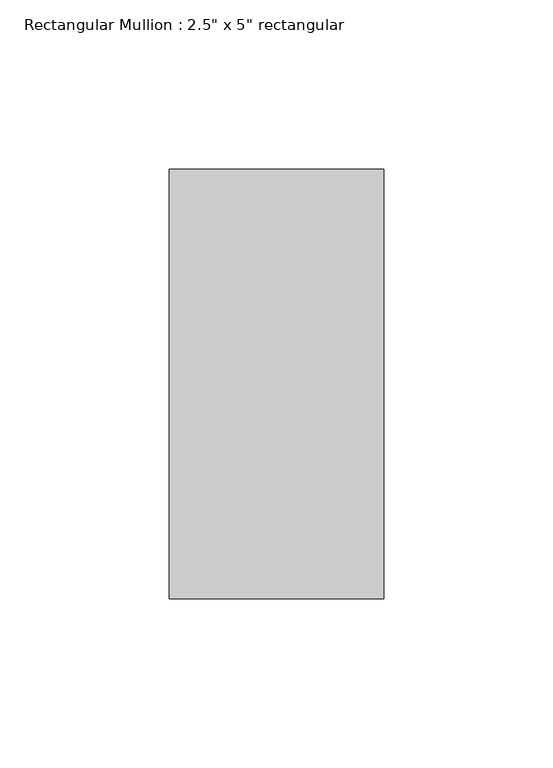
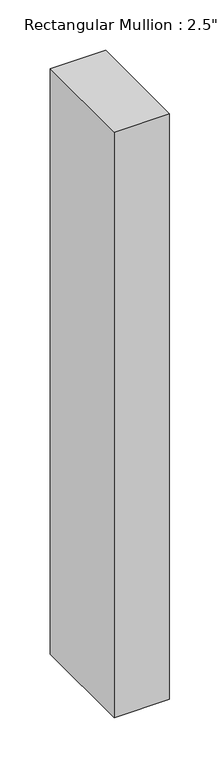
"""IFC4 building model written with IfcOpenShell, lengths in millimetres: member geometry."""

from ifc_helpers import new_model, si_unit, frame, origin, place, context, project, spatial, polyline, outline, extrude, source, transform, mapped, element, save


def member_7823a6e7(model_context):
    return source(origin(), model_context, "Body", "SweptSolid", [
        extrude(outline(polyline([(0.0, 63.5), (0.0, -63.5), (-63.5, -63.5), (-63.5, 63.5), (0.0, 63.5)])), frame((0.0, 0.0, -711.2000043), z_axis=(0.0, 0.0, 1.0), x_axis=(1.0, 0.0, 0.0)), (0.0, 0.0, 1.0), 711.2000043),
    ])


if __name__ == "__main__":
    model = new_model("IFC4")
    model_context = context("Model", 3, world=origin())
    ifc_project = project(units=[si_unit("LENGTHUNIT", "METRE", prefix="MILLI")], contexts=[model_context])
    site = spatial("IfcSite", under=ifc_project)
    building = spatial("IfcBuilding", under=site)
    placement = place(None, origin())
    member_shape = member_7823a6e7(model_context)
    element("IfcMember", 1, ObjectType="Rectangular Mullion : 2.5\" x 5\" rectangular", at=placement, inside=building, context=model_context, shape_type="MappedRepresentation", body=[
        mapped(member_shape, transform((0.0, 0.0, 0.0), x_axis=(1.0, 0.0, 0.0), y_axis=(0.0, 1.0, 0.0), z_axis=(0.0, 0.0, 1.0))),
    ])
    save(model, "model.ifc")

# Revit data of these elements
# Type "Rectangular Mullion : 2.5\" x 5\" rectangular"
#   built-in parameter 1007304 = 0.416667 (stored number, unit not read)
#   built-in parameter 1007301 = 0.104167 (stored number, unit not read)
#   built-in parameter 1007300 = 0.104167 (stored number, unit not read)
# Element 1 (IfcMember, "Rectangular Mullion : 2.5\" x 5\" rectangular")
#   Materials on its faces: "Aluminum"
# Materials
#   "Aluminum": class "Metal", colour RGB 247 247 247, transparency 0, Description = "Aluminum 6061", Cost = 0
